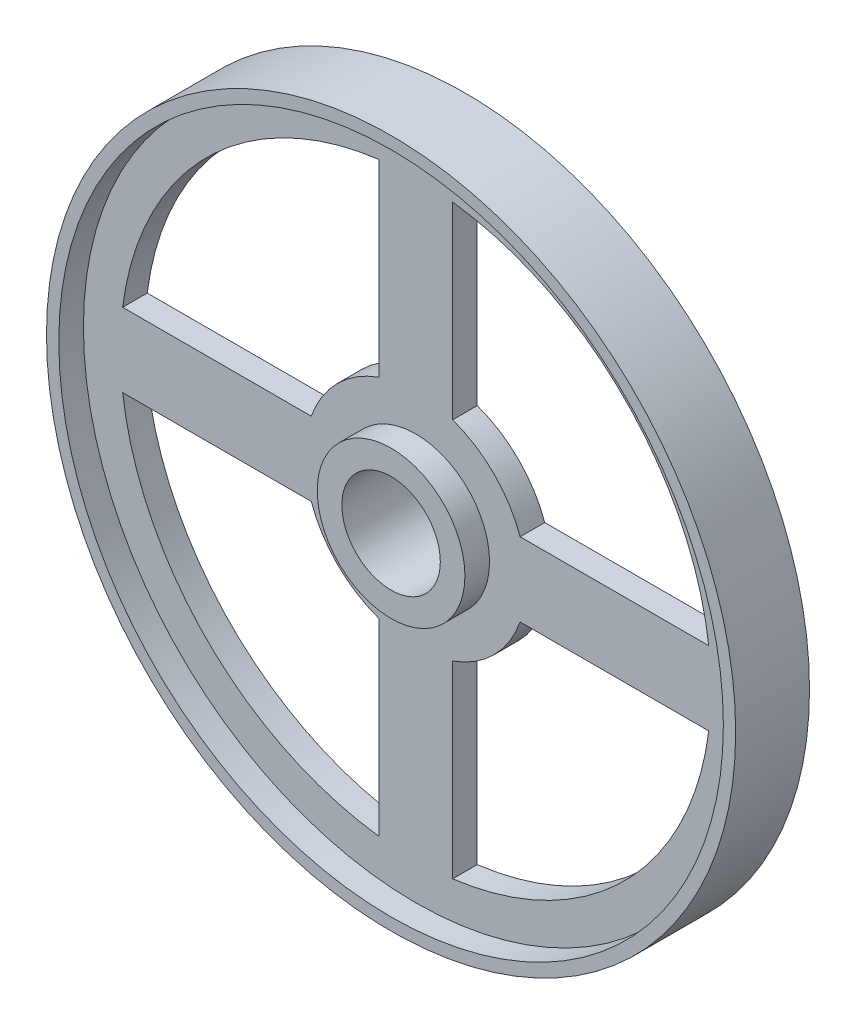
ISO-10303-21;
HEADER;
FILE_DESCRIPTION(('STEP AP214'),'2;1');
FILE_NAME('part.step','',(''),(''),'','','');
FILE_SCHEMA(('AUTOMOTIVE_DESIGN { 1 0 10303 214 1 1 1 1 }'));
ENDSEC;
DATA;
#1=APPLICATION_CONTEXT('core data for automotive mechanical design processes');
#2=APPLICATION_PROTOCOL_DEFINITION('international standard','automotive_design',2000,#1);
#3=PRODUCT_CONTEXT('',#1,'mechanical');
#4=PRODUCT('Part','Part','',(#3));
#5=PRODUCT_RELATED_PRODUCT_CATEGORY('part','',(#4));
#6=PRODUCT_DEFINITION_FORMATION('','',#4);
#7=PRODUCT_DEFINITION_CONTEXT('part definition',#1,'design');
#8=PRODUCT_DEFINITION('design','',#6,#7);
#9=PRODUCT_DEFINITION_SHAPE('','',#8);
#10=(LENGTH_UNIT() NAMED_UNIT(*) SI_UNIT(.MILLI.,.METRE.));
#11=(NAMED_UNIT(*) PLANE_ANGLE_UNIT() SI_UNIT($,.RADIAN.));
#12=(NAMED_UNIT(*) SI_UNIT($,.STERADIAN.) SOLID_ANGLE_UNIT());
#13=UNCERTAINTY_MEASURE_WITH_UNIT(LENGTH_MEASURE(1.E-05),#10,'distance_accuracy_value','');
#14=(GEOMETRIC_REPRESENTATION_CONTEXT(3) GLOBAL_UNCERTAINTY_ASSIGNED_CONTEXT((#13)) GLOBAL_UNIT_ASSIGNED_CONTEXT((#10,
#11,#12)) REPRESENTATION_CONTEXT('',''));
#15=CARTESIAN_POINT('',(0.,0.,0.));
#16=DIRECTION('',(0.,0.,1.));
#17=DIRECTION('',(1.,0.,0.));
#18=AXIS2_PLACEMENT_3D('',#15,#16,#17);
#19=CARTESIAN_POINT('',(0.,0.,0.5));
#20=DIRECTION('',(0.,0.,1.));
#21=DIRECTION('',(1.,0.,0.));
#22=AXIS2_PLACEMENT_3D('',#19,#20,#21);
#23=PLANE('',#22);
#24=DIRECTION('',(1.,0.,0.));
#25=VECTOR('',#24,1.);
#26=CARTESIAN_POINT('',(0.,0.75,0.5));
#27=LINE('',#26,#25);
#28=CARTESIAN_POINT('',(2.12132034355964,0.75,0.5));
#29=VERTEX_POINT('',#28);
#30=CARTESIAN_POINT('',(5.95294044989533,0.75,0.5));
#31=VERTEX_POINT('',#30);
#32=EDGE_CURVE('E211',#29,#31,#27,.T.);
#33=ORIENTED_EDGE('',*,*,#32,.T.);
#34=CARTESIAN_POINT('',(0.,0.,0.5));
#35=DIRECTION('',(0.,0.,1.));
#36=DIRECTION('',(1.,0.,0.));
#37=AXIS2_PLACEMENT_3D('',#34,#35,#36);
#38=CIRCLE('',#37,6.);
#39=CARTESIAN_POINT('',(0.75,5.95294044989533,0.5));
#40=VERTEX_POINT('',#39);
#41=EDGE_CURVE('E212',#31,#40,#38,.T.);
#42=ORIENTED_EDGE('',*,*,#41,.T.);
#43=DIRECTION('',(0.,1.,0.));
#44=VECTOR('',#43,1.);
#45=CARTESIAN_POINT('',(0.75,0.,0.5));
#46=LINE('',#45,#44);
#47=CARTESIAN_POINT('',(0.75,2.12132034355964,0.5));
#48=VERTEX_POINT('',#47);
#49=EDGE_CURVE('E220',#48,#40,#46,.T.);
#50=ORIENTED_EDGE('',*,*,#49,.F.);
#51=CARTESIAN_POINT('',(0.,0.,0.5));
#52=DIRECTION('',(0.,0.,-1.));
#53=DIRECTION('',(-1.,0.,0.));
#54=AXIS2_PLACEMENT_3D('',#51,#52,#53);
#55=CIRCLE('',#54,2.25);
#56=EDGE_CURVE('E169',#48,#29,#55,.T.);
#57=ORIENTED_EDGE('',*,*,#56,.T.);
#58=EDGE_LOOP('',(#33,#42,#50,#57));
#59=FACE_BOUND('',#58,.T.);
#60=CARTESIAN_POINT('',(2.12132034355964,-0.75,0.5));
#61=VERTEX_POINT('',#60);
#62=CARTESIAN_POINT('',(0.75,-2.12132034355964,0.5));
#63=VERTEX_POINT('',#62);
#64=EDGE_CURVE('E314',#61,#63,#55,.T.);
#65=ORIENTED_EDGE('',*,*,#64,.T.);
#66=DIRECTION('',(0.,1.,0.));
#67=VECTOR('',#66,1.);
#68=CARTESIAN_POINT('',(0.75,0.,0.5));
#69=LINE('',#68,#67);
#70=CARTESIAN_POINT('',(0.75,-5.95294044989533,0.5));
#71=VERTEX_POINT('',#70);
#72=EDGE_CURVE('E241',#71,#63,#69,.T.);
#73=ORIENTED_EDGE('',*,*,#72,.F.);
#74=CARTESIAN_POINT('',(5.95294044989533,-0.75,0.5));
#75=VERTEX_POINT('',#74);
#76=EDGE_CURVE('E209',#71,#75,#38,.T.);
#77=ORIENTED_EDGE('',*,*,#76,.T.);
#78=DIRECTION('',(-1.,0.,0.));
#79=VECTOR('',#78,1.);
#80=CARTESIAN_POINT('',(0.,-0.75,0.5));
#81=LINE('',#80,#79);
#82=EDGE_CURVE('E238',#75,#61,#81,.T.);
#83=ORIENTED_EDGE('',*,*,#82,.T.);
#84=EDGE_LOOP('',(#65,#73,#77,#83));
#85=FACE_BOUND('',#84,.T.);
#86=CARTESIAN_POINT('',(-0.75,-2.12132034355964,0.5));
#87=VERTEX_POINT('',#86);
#88=CARTESIAN_POINT('',(-2.12132034355964,-0.75,0.5));
#89=VERTEX_POINT('',#88);
#90=EDGE_CURVE('E171',#87,#89,#55,.T.);
#91=ORIENTED_EDGE('',*,*,#90,.T.);
#92=DIRECTION('',(-1.,0.,0.));
#93=VECTOR('',#92,1.);
#94=CARTESIAN_POINT('',(0.,-0.75,0.5));
#95=LINE('',#94,#93);
#96=CARTESIAN_POINT('',(-5.95294044989533,-0.75,0.5));
#97=VERTEX_POINT('',#96);
#98=EDGE_CURVE('E260',#89,#97,#95,.T.);
#99=ORIENTED_EDGE('',*,*,#98,.T.);
#100=CARTESIAN_POINT('',(-0.75,-5.95294044989533,0.5));
#101=VERTEX_POINT('',#100);
#102=EDGE_CURVE('E298',#97,#101,#38,.T.);
#103=ORIENTED_EDGE('',*,*,#102,.T.);
#104=DIRECTION('',(0.,-1.,0.));
#105=VECTOR('',#104,1.);
#106=CARTESIAN_POINT('',(-0.75,0.,0.5));
#107=LINE('',#106,#105);
#108=EDGE_CURVE('E264',#87,#101,#107,.T.);
#109=ORIENTED_EDGE('',*,*,#108,.F.);
#110=EDGE_LOOP('',(#91,#99,#103,#109));
#111=FACE_BOUND('',#110,.T.);
#112=CARTESIAN_POINT('',(-2.12132034355964,0.75,0.5));
#113=VERTEX_POINT('',#112);
#114=CARTESIAN_POINT('',(-0.75,2.12132034355964,0.5));
#115=VERTEX_POINT('',#114);
#116=EDGE_CURVE('E162',#113,#115,#55,.T.);
#117=ORIENTED_EDGE('',*,*,#116,.T.);
#118=DIRECTION('',(0.,-1.,0.));
#119=VECTOR('',#118,1.);
#120=CARTESIAN_POINT('',(-0.75,0.,0.5));
#121=LINE('',#120,#119);
#122=CARTESIAN_POINT('',(-0.75,5.95294044989533,0.5));
#123=VERTEX_POINT('',#122);
#124=EDGE_CURVE('E181',#123,#115,#121,.T.);
#125=ORIENTED_EDGE('',*,*,#124,.F.);
#126=CARTESIAN_POINT('',(-5.95294044989533,0.75,0.5));
#127=VERTEX_POINT('',#126);
#128=EDGE_CURVE('E179',#123,#127,#38,.T.);
#129=ORIENTED_EDGE('',*,*,#128,.T.);
#130=DIRECTION('',(1.,0.,0.));
#131=VECTOR('',#130,1.);
#132=CARTESIAN_POINT('',(0.,0.75,0.5));
#133=LINE('',#132,#131);
#134=EDGE_CURVE('E72',#127,#113,#133,.T.);
#135=ORIENTED_EDGE('',*,*,#134,.T.);
#136=EDGE_LOOP('',(#117,#125,#129,#135));
#137=FACE_BOUND('',#136,.T.);
#138=CARTESIAN_POINT('',(0.,0.,0.5));
#139=DIRECTION('',(0.,0.,-1.));
#140=DIRECTION('',(-1.,0.,0.));
#141=AXIS2_PLACEMENT_3D('',#138,#139,#140);
#142=CIRCLE('',#141,1.5);
#143=CARTESIAN_POINT('',(-1.5,0.,0.5));
#144=VERTEX_POINT('',#143);
#145=EDGE_CURVE('E54',#144,#144,#142,.T.);
#146=ORIENTED_EDGE('',*,*,#145,.F.);
#147=EDGE_LOOP('',(#146));
#148=FACE_BOUND('',#147,.T.);
#149=CARTESIAN_POINT('',(0.,0.,0.5));
#150=DIRECTION('',(0.,0.,-1.));
#151=DIRECTION('',(-1.,0.,0.));
#152=AXIS2_PLACEMENT_3D('',#149,#150,#151);
#153=CIRCLE('',#152,6.75);
#154=CARTESIAN_POINT('',(-6.75,0.,0.5));
#155=VERTEX_POINT('',#154);
#156=EDGE_CURVE('E407',#155,#155,#153,.T.);
#157=ORIENTED_EDGE('',*,*,#156,.T.);
#158=EDGE_LOOP('',(#157));
#159=FACE_BOUND('',#158,.T.);
#160=ADVANCED_FACE('F50',(#59,#85,#111,#137,#148,#159),#23,.F.);
#161=CARTESIAN_POINT('',(0.,0.,1.));
#162=DIRECTION('',(0.,0.,1.));
#163=DIRECTION('',(1.,0.,0.));
#164=AXIS2_PLACEMENT_3D('',#161,#162,#163);
#165=PLANE('',#164);
#166=CARTESIAN_POINT('',(0.,0.,1.));
#167=DIRECTION('',(0.,0.,1.));
#168=DIRECTION('',(1.,0.,0.));
#169=AXIS2_PLACEMENT_3D('',#166,#167,#168);
#170=CIRCLE('',#169,2.25);
#171=CARTESIAN_POINT('',(2.12132034355964,0.75,1.));
#172=VERTEX_POINT('',#171);
#173=CARTESIAN_POINT('',(0.75,2.12132034355964,1.));
#174=VERTEX_POINT('',#173);
#175=EDGE_CURVE('E313',#172,#174,#170,.T.);
#176=ORIENTED_EDGE('',*,*,#175,.T.);
#177=DIRECTION('',(0.,1.,0.));
#178=VECTOR('',#177,1.);
#179=CARTESIAN_POINT('',(0.75,0.,1.));
#180=LINE('',#179,#178);
#181=CARTESIAN_POINT('',(0.75,5.95294044989533,1.));
#182=VERTEX_POINT('',#181);
#183=EDGE_CURVE('E216',#174,#182,#180,.T.);
#184=ORIENTED_EDGE('',*,*,#183,.T.);
#185=CARTESIAN_POINT('',(0.,0.,1.));
#186=DIRECTION('',(0.,0.,1.));
#187=DIRECTION('',(1.,0.,0.));
#188=AXIS2_PLACEMENT_3D('',#185,#186,#187);
#189=CIRCLE('',#188,6.);
#190=CARTESIAN_POINT('',(5.95294044989533,0.75,1.));
#191=VERTEX_POINT('',#190);
#192=EDGE_CURVE('E207',#191,#182,#189,.T.);
#193=ORIENTED_EDGE('',*,*,#192,.F.);
#194=DIRECTION('',(1.,0.,0.));
#195=VECTOR('',#194,1.);
#196=CARTESIAN_POINT('',(0.,0.75,1.));
#197=LINE('',#196,#195);
#198=EDGE_CURVE('E223',#172,#191,#197,.T.);
#199=ORIENTED_EDGE('',*,*,#198,.F.);
#200=EDGE_LOOP('',(#176,#184,#193,#199));
#201=FACE_BOUND('',#200,.T.);
#202=DIRECTION('',(0.,1.,0.));
#203=VECTOR('',#202,1.);
#204=CARTESIAN_POINT('',(0.75,0.,1.));
#205=LINE('',#204,#203);
#206=CARTESIAN_POINT('',(0.75,-5.95294044989533,1.));
#207=VERTEX_POINT('',#206);
#208=CARTESIAN_POINT('',(0.75,-2.12132034355964,1.));
#209=VERTEX_POINT('',#208);
#210=EDGE_CURVE('E245',#207,#209,#205,.T.);
#211=ORIENTED_EDGE('',*,*,#210,.T.);
#212=CARTESIAN_POINT('',(2.12132034355964,-0.75,1.));
#213=VERTEX_POINT('',#212);
#214=EDGE_CURVE('E64',#209,#213,#170,.T.);
#215=ORIENTED_EDGE('',*,*,#214,.T.);
#216=DIRECTION('',(-1.,0.,0.));
#217=VECTOR('',#216,1.);
#218=CARTESIAN_POINT('',(0.,-0.75,1.));
#219=LINE('',#218,#217);
#220=CARTESIAN_POINT('',(5.95294044989533,-0.75,1.));
#221=VERTEX_POINT('',#220);
#222=EDGE_CURVE('E246',#221,#213,#219,.T.);
#223=ORIENTED_EDGE('',*,*,#222,.F.);
#224=EDGE_CURVE('E208',#207,#221,#189,.T.);
#225=ORIENTED_EDGE('',*,*,#224,.F.);
#226=EDGE_LOOP('',(#211,#215,#223,#225));
#227=FACE_BOUND('',#226,.T.);
#228=DIRECTION('',(-1.,0.,0.));
#229=VECTOR('',#228,1.);
#230=CARTESIAN_POINT('',(0.,-0.75,1.));
#231=LINE('',#230,#229);
#232=CARTESIAN_POINT('',(-2.12132034355964,-0.75,1.));
#233=VERTEX_POINT('',#232);
#234=CARTESIAN_POINT('',(-5.95294044989533,-0.75,1.));
#235=VERTEX_POINT('',#234);
#236=EDGE_CURVE('E267',#233,#235,#231,.T.);
#237=ORIENTED_EDGE('',*,*,#236,.F.);
#238=CARTESIAN_POINT('',(-0.75,-2.12132034355964,1.));
#239=VERTEX_POINT('',#238);
#240=EDGE_CURVE('E290',#233,#239,#170,.T.);
#241=ORIENTED_EDGE('',*,*,#240,.T.);
#242=DIRECTION('',(0.,-1.,0.));
#243=VECTOR('',#242,1.);
#244=CARTESIAN_POINT('',(-0.75,0.,1.));
#245=LINE('',#244,#243);
#246=CARTESIAN_POINT('',(-0.75,-5.95294044989533,1.));
#247=VERTEX_POINT('',#246);
#248=EDGE_CURVE('E265',#239,#247,#245,.T.);
#249=ORIENTED_EDGE('',*,*,#248,.T.);
#250=EDGE_CURVE('E210',#235,#247,#189,.T.);
#251=ORIENTED_EDGE('',*,*,#250,.F.);
#252=EDGE_LOOP('',(#237,#241,#249,#251));
#253=FACE_BOUND('',#252,.T.);
#254=DIRECTION('',(0.,-1.,0.));
#255=VECTOR('',#254,1.);
#256=CARTESIAN_POINT('',(-0.75,0.,1.));
#257=LINE('',#256,#255);
#258=CARTESIAN_POINT('',(-0.75,5.95294044989533,1.));
#259=VERTEX_POINT('',#258);
#260=CARTESIAN_POINT('',(-0.75,2.12132034355964,1.));
#261=VERTEX_POINT('',#260);
#262=EDGE_CURVE('E185',#259,#261,#257,.T.);
#263=ORIENTED_EDGE('',*,*,#262,.T.);
#264=CARTESIAN_POINT('',(-2.12132034355964,0.75,1.));
#265=VERTEX_POINT('',#264);
#266=EDGE_CURVE('E203',#261,#265,#170,.T.);
#267=ORIENTED_EDGE('',*,*,#266,.T.);
#268=DIRECTION('',(1.,0.,0.));
#269=VECTOR('',#268,1.);
#270=CARTESIAN_POINT('',(0.,0.75,1.));
#271=LINE('',#270,#269);
#272=CARTESIAN_POINT('',(-5.95294044989533,0.75,1.));
#273=VERTEX_POINT('',#272);
#274=EDGE_CURVE('E174',#273,#265,#271,.T.);
#275=ORIENTED_EDGE('',*,*,#274,.F.);
#276=EDGE_CURVE('E202',#259,#273,#189,.T.);
#277=ORIENTED_EDGE('',*,*,#276,.F.);
#278=EDGE_LOOP('',(#263,#267,#275,#277));
#279=FACE_BOUND('',#278,.T.);
#280=CARTESIAN_POINT('',(0.,0.,1.));
#281=DIRECTION('',(0.,0.,1.));
#282=DIRECTION('',(1.,0.,0.));
#283=AXIS2_PLACEMENT_3D('',#280,#281,#282);
#284=CIRCLE('',#283,1.5);
#285=CARTESIAN_POINT('',(1.5,0.,1.));
#286=VERTEX_POINT('',#285);
#287=EDGE_CURVE('E426',#286,#286,#284,.T.);
#288=ORIENTED_EDGE('',*,*,#287,.F.);
#289=EDGE_LOOP('',(#288));
#290=FACE_BOUND('',#289,.T.);
#291=CARTESIAN_POINT('',(0.,0.,1.));
#292=DIRECTION('',(0.,0.,1.));
#293=DIRECTION('',(1.,0.,0.));
#294=AXIS2_PLACEMENT_3D('',#291,#292,#293);
#295=CIRCLE('',#294,6.75);
#296=CARTESIAN_POINT('',(6.75,0.,1.));
#297=VERTEX_POINT('',#296);
#298=EDGE_CURVE('E11',#297,#297,#295,.F.);
#299=ORIENTED_EDGE('',*,*,#298,.F.);
#300=EDGE_LOOP('',(#299));
#301=FACE_BOUND('',#300,.T.);
#302=ADVANCED_FACE('F196',(#201,#227,#253,#279,#290,#301),#165,.T.);
#303=CARTESIAN_POINT('',(0.,0.,0.5));
#304=DIRECTION('',(0.,0.,-1.));
#305=DIRECTION('',(-1.,0.,0.));
#306=AXIS2_PLACEMENT_3D('',#303,#304,#305);
#307=CYLINDRICAL_SURFACE('',#306,2.25);
#308=ORIENTED_EDGE('',*,*,#116,.F.);
#309=DIRECTION('',(0.,0.,1.));
#310=VECTOR('',#309,1.);
#311=CARTESIAN_POINT('',(-2.12132034355964,0.75,0.5));
#312=LINE('',#311,#310);
#313=EDGE_CURVE('E161',#113,#265,#312,.T.);
#314=ORIENTED_EDGE('',*,*,#313,.T.);
#315=ORIENTED_EDGE('',*,*,#266,.F.);
#316=DIRECTION('',(0.,0.,1.));
#317=VECTOR('',#316,1.);
#318=CARTESIAN_POINT('',(-0.75,2.12132034355964,0.5));
#319=LINE('',#318,#317);
#320=EDGE_CURVE('E164',#115,#261,#319,.T.);
#321=ORIENTED_EDGE('',*,*,#320,.F.);
#322=EDGE_LOOP('',(#308,#314,#315,#321));
#323=FACE_BOUND('',#322,.T.);
#324=ADVANCED_FACE('F47',(#323),#307,.T.);
#325=ORIENTED_EDGE('',*,*,#56,.F.);
#326=DIRECTION('',(0.,0.,1.));
#327=VECTOR('',#326,1.);
#328=CARTESIAN_POINT('',(0.75,2.12132034355964,0.5));
#329=LINE('',#328,#327);
#330=EDGE_CURVE('E193',#48,#174,#329,.T.);
#331=ORIENTED_EDGE('',*,*,#330,.T.);
#332=ORIENTED_EDGE('',*,*,#175,.F.);
#333=DIRECTION('',(0.,0.,1.));
#334=VECTOR('',#333,1.);
#335=CARTESIAN_POINT('',(2.12132034355964,0.75,0.5));
#336=LINE('',#335,#334);
#337=EDGE_CURVE('E225',#29,#172,#336,.T.);
#338=ORIENTED_EDGE('',*,*,#337,.F.);
#339=EDGE_LOOP('',(#325,#331,#332,#338));
#340=FACE_BOUND('',#339,.T.);
#341=ADVANCED_FACE('F315',(#340),#307,.T.);
#342=ORIENTED_EDGE('',*,*,#64,.F.);
#343=DIRECTION('',(0.,0.,1.));
#344=VECTOR('',#343,1.);
#345=CARTESIAN_POINT('',(2.12132034355964,-0.75,0.5));
#346=LINE('',#345,#344);
#347=EDGE_CURVE('E251',#61,#213,#346,.T.);
#348=ORIENTED_EDGE('',*,*,#347,.T.);
#349=ORIENTED_EDGE('',*,*,#214,.F.);
#350=DIRECTION('',(0.,0.,1.));
#351=VECTOR('',#350,1.);
#352=CARTESIAN_POINT('',(0.75,-2.12132034355964,0.5));
#353=LINE('',#352,#351);
#354=EDGE_CURVE('E252',#63,#209,#353,.T.);
#355=ORIENTED_EDGE('',*,*,#354,.F.);
#356=EDGE_LOOP('',(#342,#348,#349,#355));
#357=FACE_BOUND('',#356,.T.);
#358=ADVANCED_FACE('F545',(#357),#307,.T.);
#359=ORIENTED_EDGE('',*,*,#90,.F.);
#360=DIRECTION('',(0.,0.,1.));
#361=VECTOR('',#360,1.);
#362=CARTESIAN_POINT('',(-0.75,-2.12132034355964,0.5));
#363=LINE('',#362,#361);
#364=EDGE_CURVE('E247',#87,#239,#363,.T.);
#365=ORIENTED_EDGE('',*,*,#364,.T.);
#366=ORIENTED_EDGE('',*,*,#240,.F.);
#367=DIRECTION('',(0.,0.,1.));
#368=VECTOR('',#367,1.);
#369=CARTESIAN_POINT('',(-2.12132034355964,-0.75,0.5));
#370=LINE('',#369,#368);
#371=EDGE_CURVE('E189',#89,#233,#370,.T.);
#372=ORIENTED_EDGE('',*,*,#371,.F.);
#373=EDGE_LOOP('',(#359,#365,#366,#372));
#374=FACE_BOUND('',#373,.T.);
#375=ADVANCED_FACE('F331',(#374),#307,.T.);
#376=CARTESIAN_POINT('',(-0.75,0.,0.5));
#377=DIRECTION('',(-1.,0.,0.));
#378=DIRECTION('',(0.,0.,1.));
#379=AXIS2_PLACEMENT_3D('',#376,#377,#378);
#380=PLANE('',#379);
#381=ORIENTED_EDGE('',*,*,#262,.F.);
#382=DIRECTION('',(0.,0.,1.));
#383=VECTOR('',#382,1.);
#384=CARTESIAN_POINT('',(-0.75,5.95294044989533,0.5));
#385=LINE('',#384,#383);
#386=EDGE_CURVE('E192',#123,#259,#385,.T.);
#387=ORIENTED_EDGE('',*,*,#386,.F.);
#388=ORIENTED_EDGE('',*,*,#124,.T.);
#389=ORIENTED_EDGE('',*,*,#320,.T.);
#390=EDGE_LOOP('',(#381,#387,#388,#389));
#391=FACE_BOUND('',#390,.T.);
#392=ADVANCED_FACE('F338',(#391),#380,.T.);
#393=CARTESIAN_POINT('',(0.,0.75,0.5));
#394=DIRECTION('',(0.,-1.,0.));
#395=DIRECTION('',(0.,0.,-1.));
#396=AXIS2_PLACEMENT_3D('',#393,#394,#395);
#397=PLANE('',#396);
#398=ORIENTED_EDGE('',*,*,#274,.T.);
#399=ORIENTED_EDGE('',*,*,#313,.F.);
#400=ORIENTED_EDGE('',*,*,#134,.F.);
#401=DIRECTION('',(0.,0.,1.));
#402=VECTOR('',#401,1.);
#403=CARTESIAN_POINT('',(-5.95294044989533,0.75,0.5));
#404=LINE('',#403,#402);
#405=EDGE_CURVE('E176',#127,#273,#404,.T.);
#406=ORIENTED_EDGE('',*,*,#405,.T.);
#407=EDGE_LOOP('',(#398,#399,#400,#406));
#408=FACE_BOUND('',#407,.T.);
#409=ADVANCED_FACE('F173',(#408),#397,.F.);
#410=CARTESIAN_POINT('',(0.75,0.,0.5));
#411=DIRECTION('',(1.,0.,0.));
#412=DIRECTION('',(0.,0.,-1.));
#413=AXIS2_PLACEMENT_3D('',#410,#411,#412);
#414=PLANE('',#413);
#415=ORIENTED_EDGE('',*,*,#183,.F.);
#416=ORIENTED_EDGE('',*,*,#330,.F.);
#417=ORIENTED_EDGE('',*,*,#49,.T.);
#418=DIRECTION('',(0.,0.,1.));
#419=VECTOR('',#418,1.);
#420=CARTESIAN_POINT('',(0.75,5.95294044989533,0.5));
#421=LINE('',#420,#419);
#422=EDGE_CURVE('E233',#40,#182,#421,.T.);
#423=ORIENTED_EDGE('',*,*,#422,.T.);
#424=EDGE_LOOP('',(#415,#416,#417,#423));
#425=FACE_BOUND('',#424,.T.);
#426=ADVANCED_FACE('F309',(#425),#414,.T.);
#427=CARTESIAN_POINT('',(0.,0.75,0.5));
#428=DIRECTION('',(0.,-1.,0.));
#429=DIRECTION('',(0.,0.,-1.));
#430=AXIS2_PLACEMENT_3D('',#427,#428,#429);
#431=PLANE('',#430);
#432=ORIENTED_EDGE('',*,*,#198,.T.);
#433=DIRECTION('',(0.,0.,1.));
#434=VECTOR('',#433,1.);
#435=CARTESIAN_POINT('',(5.95294044989533,0.75,0.5));
#436=LINE('',#435,#434);
#437=EDGE_CURVE('E234',#31,#191,#436,.T.);
#438=ORIENTED_EDGE('',*,*,#437,.F.);
#439=ORIENTED_EDGE('',*,*,#32,.F.);
#440=ORIENTED_EDGE('',*,*,#337,.T.);
#441=EDGE_LOOP('',(#432,#438,#439,#440));
#442=FACE_BOUND('',#441,.T.);
#443=ADVANCED_FACE('F353',(#442),#431,.F.);
#444=CARTESIAN_POINT('',(0.75,0.,0.5));
#445=DIRECTION('',(1.,0.,0.));
#446=DIRECTION('',(0.,0.,-1.));
#447=AXIS2_PLACEMENT_3D('',#444,#445,#446);
#448=PLANE('',#447);
#449=ORIENTED_EDGE('',*,*,#210,.F.);
#450=DIRECTION('',(0.,0.,1.));
#451=VECTOR('',#450,1.);
#452=CARTESIAN_POINT('',(0.75,-5.95294044989533,0.5));
#453=LINE('',#452,#451);
#454=EDGE_CURVE('E228',#71,#207,#453,.T.);
#455=ORIENTED_EDGE('',*,*,#454,.F.);
#456=ORIENTED_EDGE('',*,*,#72,.T.);
#457=ORIENTED_EDGE('',*,*,#354,.T.);
#458=EDGE_LOOP('',(#449,#455,#456,#457));
#459=FACE_BOUND('',#458,.T.);
#460=ADVANCED_FACE('F348',(#459),#448,.T.);
#461=CARTESIAN_POINT('',(0.,-0.75,0.5));
#462=DIRECTION('',(0.,1.,0.));
#463=DIRECTION('',(0.,0.,1.));
#464=AXIS2_PLACEMENT_3D('',#461,#462,#463);
#465=PLANE('',#464);
#466=ORIENTED_EDGE('',*,*,#222,.T.);
#467=ORIENTED_EDGE('',*,*,#347,.F.);
#468=ORIENTED_EDGE('',*,*,#82,.F.);
#469=DIRECTION('',(0.,0.,1.));
#470=VECTOR('',#469,1.);
#471=CARTESIAN_POINT('',(5.95294044989533,-0.75,0.5));
#472=LINE('',#471,#470);
#473=EDGE_CURVE('E244',#75,#221,#472,.T.);
#474=ORIENTED_EDGE('',*,*,#473,.T.);
#475=EDGE_LOOP('',(#466,#467,#468,#474));
#476=FACE_BOUND('',#475,.T.);
#477=ADVANCED_FACE('F327',(#476),#465,.F.);
#478=CARTESIAN_POINT('',(-0.75,0.,0.5));
#479=DIRECTION('',(-1.,0.,0.));
#480=DIRECTION('',(0.,0.,1.));
#481=AXIS2_PLACEMENT_3D('',#478,#479,#480);
#482=PLANE('',#481);
#483=ORIENTED_EDGE('',*,*,#248,.F.);
#484=ORIENTED_EDGE('',*,*,#364,.F.);
#485=ORIENTED_EDGE('',*,*,#108,.T.);
#486=DIRECTION('',(0.,0.,1.));
#487=VECTOR('',#486,1.);
#488=CARTESIAN_POINT('',(-0.75,-5.95294044989533,0.5));
#489=LINE('',#488,#487);
#490=EDGE_CURVE('E275',#101,#247,#489,.T.);
#491=ORIENTED_EDGE('',*,*,#490,.T.);
#492=EDGE_LOOP('',(#483,#484,#485,#491));
#493=FACE_BOUND('',#492,.T.);
#494=ADVANCED_FACE('F292',(#493),#482,.T.);
#495=CARTESIAN_POINT('',(0.,-0.75,0.5));
#496=DIRECTION('',(0.,1.,0.));
#497=DIRECTION('',(0.,0.,1.));
#498=AXIS2_PLACEMENT_3D('',#495,#496,#497);
#499=PLANE('',#498);
#500=ORIENTED_EDGE('',*,*,#236,.T.);
#501=DIRECTION('',(0.,0.,1.));
#502=VECTOR('',#501,1.);
#503=CARTESIAN_POINT('',(-5.95294044989533,-0.75,0.5));
#504=LINE('',#503,#502);
#505=EDGE_CURVE('E274',#97,#235,#504,.T.);
#506=ORIENTED_EDGE('',*,*,#505,.F.);
#507=ORIENTED_EDGE('',*,*,#98,.F.);
#508=ORIENTED_EDGE('',*,*,#371,.T.);
#509=EDGE_LOOP('',(#500,#506,#507,#508));
#510=FACE_BOUND('',#509,.T.);
#511=ADVANCED_FACE('F281',(#510),#499,.F.);
#512=CARTESIAN_POINT('',(0.,0.,0.5));
#513=DIRECTION('',(0.,0.,1.));
#514=DIRECTION('',(1.,0.,0.));
#515=AXIS2_PLACEMENT_3D('',#512,#513,#514);
#516=CYLINDRICAL_SURFACE('',#515,6.);
#517=ORIENTED_EDGE('',*,*,#386,.T.);
#518=ORIENTED_EDGE('',*,*,#276,.T.);
#519=ORIENTED_EDGE('',*,*,#405,.F.);
#520=ORIENTED_EDGE('',*,*,#128,.F.);
#521=EDGE_LOOP('',(#517,#518,#519,#520));
#522=FACE_BOUND('',#521,.T.);
#523=ADVANCED_FACE('F204',(#522),#516,.F.);
#524=ORIENTED_EDGE('',*,*,#422,.F.);
#525=ORIENTED_EDGE('',*,*,#41,.F.);
#526=ORIENTED_EDGE('',*,*,#437,.T.);
#527=ORIENTED_EDGE('',*,*,#192,.T.);
#528=EDGE_LOOP('',(#524,#525,#526,#527));
#529=FACE_BOUND('',#528,.T.);
#530=ADVANCED_FACE('F573',(#529),#516,.F.);
#531=ORIENTED_EDGE('',*,*,#454,.T.);
#532=ORIENTED_EDGE('',*,*,#224,.T.);
#533=ORIENTED_EDGE('',*,*,#473,.F.);
#534=ORIENTED_EDGE('',*,*,#76,.F.);
#535=EDGE_LOOP('',(#531,#532,#533,#534));
#536=FACE_BOUND('',#535,.T.);
#537=ADVANCED_FACE('F324',(#536),#516,.F.);
#538=ORIENTED_EDGE('',*,*,#490,.F.);
#539=ORIENTED_EDGE('',*,*,#102,.F.);
#540=ORIENTED_EDGE('',*,*,#505,.T.);
#541=ORIENTED_EDGE('',*,*,#250,.T.);
#542=EDGE_LOOP('',(#538,#539,#540,#541));
#543=FACE_BOUND('',#542,.T.);
#544=ADVANCED_FACE('F289',(#543),#516,.F.);
#545=CARTESIAN_POINT('',(0.,0.,0.));
#546=DIRECTION('',(0.,0.,1.));
#547=DIRECTION('',(1.,0.,0.));
#548=AXIS2_PLACEMENT_3D('',#545,#546,#547);
#549=CYLINDRICAL_SURFACE('',#548,1.5);
#550=CARTESIAN_POINT('',(0.,0.,0.));
#551=DIRECTION('',(0.,0.,-1.));
#552=DIRECTION('',(-1.,0.,0.));
#553=AXIS2_PLACEMENT_3D('',#550,#551,#552);
#554=CIRCLE('',#553,1.5);
#555=CARTESIAN_POINT('',(-1.5,0.,0.));
#556=VERTEX_POINT('',#555);
#557=EDGE_CURVE('E435',#556,#556,#554,.T.);
#558=ORIENTED_EDGE('',*,*,#557,.F.);
#559=EDGE_LOOP('',(#558));
#560=FACE_BOUND('',#559,.T.);
#561=ORIENTED_EDGE('',*,*,#145,.T.);
#562=EDGE_LOOP('',(#561));
#563=FACE_BOUND('',#562,.T.);
#564=ADVANCED_FACE('F365',(#560,#563),#549,.T.);
#565=CARTESIAN_POINT('',(0.,0.,0.));
#566=DIRECTION('',(0.,0.,-1.));
#567=DIRECTION('',(-1.,0.,0.));
#568=AXIS2_PLACEMENT_3D('',#565,#566,#567);
#569=PLANE('',#568);
#570=CARTESIAN_POINT('',(0.,0.,0.));
#571=DIRECTION('',(0.,0.,-1.));
#572=DIRECTION('',(-1.,0.,0.));
#573=AXIS2_PLACEMENT_3D('',#570,#571,#572);
#574=CIRCLE('',#573,1.);
#575=CARTESIAN_POINT('',(-1.,0.,0.));
#576=VERTEX_POINT('',#575);
#577=EDGE_CURVE('E424',#576,#576,#574,.T.);
#578=ORIENTED_EDGE('',*,*,#577,.F.);
#579=EDGE_LOOP('',(#578));
#580=FACE_BOUND('',#579,.T.);
#581=ORIENTED_EDGE('',*,*,#557,.T.);
#582=EDGE_LOOP('',(#581));
#583=FACE_BOUND('',#582,.T.);
#584=ADVANCED_FACE('F362',(#580,#583),#569,.T.);
#585=CARTESIAN_POINT('',(0.,0.,1.5));
#586=DIRECTION('',(0.,0.,-1.));
#587=DIRECTION('',(-1.,0.,0.));
#588=AXIS2_PLACEMENT_3D('',#585,#586,#587);
#589=CYLINDRICAL_SURFACE('',#588,1.5);
#590=CARTESIAN_POINT('',(0.,0.,1.5));
#591=DIRECTION('',(0.,0.,1.));
#592=DIRECTION('',(1.,0.,0.));
#593=AXIS2_PLACEMENT_3D('',#590,#591,#592);
#594=CIRCLE('',#593,1.5);
#595=CARTESIAN_POINT('',(1.5,0.,1.5));
#596=VERTEX_POINT('',#595);
#597=EDGE_CURVE('E429',#596,#596,#594,.T.);
#598=ORIENTED_EDGE('',*,*,#597,.F.);
#599=EDGE_LOOP('',(#598));
#600=FACE_BOUND('',#599,.T.);
#601=ORIENTED_EDGE('',*,*,#287,.T.);
#602=EDGE_LOOP('',(#601));
#603=FACE_BOUND('',#602,.T.);
#604=ADVANCED_FACE('F367',(#600,#603),#589,.T.);
#605=CARTESIAN_POINT('',(0.,0.,1.5));
#606=DIRECTION('',(0.,0.,1.));
#607=DIRECTION('',(1.,0.,0.));
#608=AXIS2_PLACEMENT_3D('',#605,#606,#607);
#609=PLANE('',#608);
#610=CARTESIAN_POINT('',(0.,0.,1.5));
#611=DIRECTION('',(0.,0.,1.));
#612=DIRECTION('',(1.,0.,0.));
#613=AXIS2_PLACEMENT_3D('',#610,#611,#612);
#614=CIRCLE('',#613,1.);
#615=CARTESIAN_POINT('',(1.,0.,1.5));
#616=VERTEX_POINT('',#615);
#617=EDGE_CURVE('E422',#616,#616,#614,.T.);
#618=ORIENTED_EDGE('',*,*,#617,.F.);
#619=EDGE_LOOP('',(#618));
#620=FACE_BOUND('',#619,.T.);
#621=ORIENTED_EDGE('',*,*,#597,.T.);
#622=EDGE_LOOP('',(#621));
#623=FACE_BOUND('',#622,.T.);
#624=ADVANCED_FACE('F373',(#620,#623),#609,.T.);
#625=CARTESIAN_POINT('',(0.,0.,-8.5));
#626=DIRECTION('',(0.,0.,1.));
#627=DIRECTION('',(1.,0.,0.));
#628=AXIS2_PLACEMENT_3D('',#625,#626,#627);
#629=CYLINDRICAL_SURFACE('',#628,1.);
#630=ORIENTED_EDGE('',*,*,#577,.T.);
#631=EDGE_LOOP('',(#630));
#632=FACE_BOUND('',#631,.T.);
#633=ORIENTED_EDGE('',*,*,#617,.T.);
#634=EDGE_LOOP('',(#633));
#635=FACE_BOUND('',#634,.T.);
#636=ADVANCED_FACE('F380',(#632,#635),#629,.F.);
#637=CARTESIAN_POINT('',(0.,0.,0.5));
#638=DIRECTION('',(0.,0.,1.));
#639=DIRECTION('',(1.,0.,0.));
#640=AXIS2_PLACEMENT_3D('',#637,#638,#639);
#641=CYLINDRICAL_SURFACE('',#640,7.);
#642=CARTESIAN_POINT('',(0.,0.,1.5));
#643=DIRECTION('',(0.,0.,1.));
#644=DIRECTION('',(1.,0.,0.));
#645=AXIS2_PLACEMENT_3D('',#642,#643,#644);
#646=CIRCLE('',#645,7.);
#647=CARTESIAN_POINT('',(7.,0.,1.5));
#648=VERTEX_POINT('',#647);
#649=EDGE_CURVE('E419',#648,#648,#646,.T.);
#650=ORIENTED_EDGE('',*,*,#649,.F.);
#651=EDGE_LOOP('',(#650));
#652=FACE_BOUND('',#651,.T.);
#653=CARTESIAN_POINT('',(0.,0.,0.));
#654=DIRECTION('',(0.,0.,-1.));
#655=DIRECTION('',(-1.,0.,0.));
#656=AXIS2_PLACEMENT_3D('',#653,#654,#655);
#657=CIRCLE('',#656,7.);
#658=CARTESIAN_POINT('',(-7.,0.,0.));
#659=VERTEX_POINT('',#658);
#660=EDGE_CURVE('E412',#659,#659,#657,.T.);
#661=ORIENTED_EDGE('',*,*,#660,.F.);
#662=EDGE_LOOP('',(#661));
#663=FACE_BOUND('',#662,.T.);
#664=ADVANCED_FACE('F382',(#652,#663),#641,.T.);
#665=CARTESIAN_POINT('',(0.,0.,1.5));
#666=DIRECTION('',(0.,0.,1.));
#667=DIRECTION('',(1.,0.,0.));
#668=AXIS2_PLACEMENT_3D('',#665,#666,#667);
#669=PLANE('',#668);
#670=ORIENTED_EDGE('',*,*,#649,.T.);
#671=EDGE_LOOP('',(#670));
#672=FACE_BOUND('',#671,.T.);
#673=CARTESIAN_POINT('',(0.,0.,1.5));
#674=DIRECTION('',(0.,0.,1.));
#675=DIRECTION('',(1.,0.,0.));
#676=AXIS2_PLACEMENT_3D('',#673,#674,#675);
#677=CIRCLE('',#676,6.75);
#678=CARTESIAN_POINT('',(6.75,0.,1.5));
#679=VERTEX_POINT('',#678);
#680=EDGE_CURVE('E417',#679,#679,#677,.T.);
#681=ORIENTED_EDGE('',*,*,#680,.F.);
#682=EDGE_LOOP('',(#681));
#683=FACE_BOUND('',#682,.T.);
#684=ADVANCED_FACE('F383',(#672,#683),#669,.T.);
#685=CARTESIAN_POINT('',(0.,0.,1.5));
#686=DIRECTION('',(0.,0.,-1.));
#687=DIRECTION('',(-1.,0.,0.));
#688=AXIS2_PLACEMENT_3D('',#685,#686,#687);
#689=CYLINDRICAL_SURFACE('',#688,6.75);
#690=ORIENTED_EDGE('',*,*,#680,.T.);
#691=EDGE_LOOP('',(#690));
#692=FACE_BOUND('',#691,.T.);
#693=ORIENTED_EDGE('',*,*,#298,.T.);
#694=EDGE_LOOP('',(#693));
#695=FACE_BOUND('',#694,.T.);
#696=ADVANCED_FACE('F387',(#692,#695),#689,.F.);
#697=CARTESIAN_POINT('',(0.,0.,0.));
#698=DIRECTION('',(0.,0.,-1.));
#699=DIRECTION('',(-1.,0.,0.));
#700=AXIS2_PLACEMENT_3D('',#697,#698,#699);
#701=PLANE('',#700);
#702=ORIENTED_EDGE('',*,*,#660,.T.);
#703=EDGE_LOOP('',(#702));
#704=FACE_BOUND('',#703,.T.);
#705=CARTESIAN_POINT('',(0.,0.,0.));
#706=DIRECTION('',(0.,0.,-1.));
#707=DIRECTION('',(-1.,0.,0.));
#708=AXIS2_PLACEMENT_3D('',#705,#706,#707);
#709=CIRCLE('',#708,6.75);
#710=CARTESIAN_POINT('',(-6.75,0.,0.));
#711=VERTEX_POINT('',#710);
#712=EDGE_CURVE('E403',#711,#711,#709,.T.);
#713=ORIENTED_EDGE('',*,*,#712,.F.);
#714=EDGE_LOOP('',(#713));
#715=FACE_BOUND('',#714,.T.);
#716=ADVANCED_FACE('F394',(#704,#715),#701,.T.);
#717=CARTESIAN_POINT('',(0.,0.,0.));
#718=DIRECTION('',(0.,0.,1.));
#719=DIRECTION('',(1.,0.,0.));
#720=AXIS2_PLACEMENT_3D('',#717,#718,#719);
#721=CYLINDRICAL_SURFACE('',#720,6.75);
#722=ORIENTED_EDGE('',*,*,#712,.T.);
#723=EDGE_LOOP('',(#722));
#724=FACE_BOUND('',#723,.T.);
#725=ORIENTED_EDGE('',*,*,#156,.F.);
#726=EDGE_LOOP('',(#725));
#727=FACE_BOUND('',#726,.T.);
#728=ADVANCED_FACE('F397',(#724,#727),#721,.F.);
#729=CLOSED_SHELL('',(#160,#302,#324,#341,#358,#375,#392,#409,#426,#443,#460,#477,#494,#511,
#523,#530,#537,#544,#564,#584,#604,#624,#636,#664,#684,#696,#716,#728));
#730=MANIFOLD_SOLID_BREP('B2',#729);
#731=ADVANCED_BREP_SHAPE_REPRESENTATION('',(#18,#730),#14);
#732=SHAPE_DEFINITION_REPRESENTATION(#9,#731);
ENDSEC;
END-ISO-10303-21;
